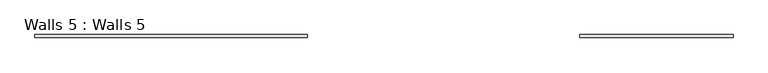
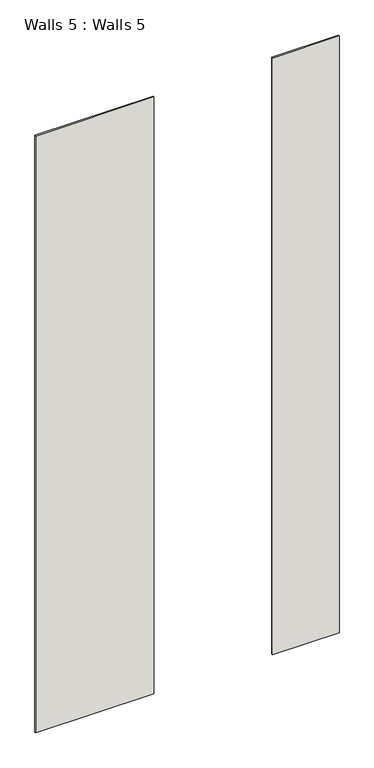
"""IFC4 building model written with IfcOpenShell, lengths in millimetres: wall geometry, Walls 5 : Walls 5."""

from ifc_helpers import new_model, si_unit, frame, origin, place, context, project, spatial, polyline, outline, extrude, source, transform, mapped, element, save


def walls_5_walls_5_43feafce(model_context):
    return source(origin(), model_context, "Body", "SweptSolid", [
        extrude(outline(polyline([(3838.3430349, 426.1055142), (2517.5430349, 426.1055142), (2517.5430349, 451.5055142), (3838.3430349, 451.5055142), (3838.3430349, 426.1055142)])), frame((0.0, 0.0, 2743.2), z_axis=(0.0, 0.0, 1.0), x_axis=(1.0, 0.0, 0.0)), (0.0, 0.0, 1.0), 12490.45),
        extrude(outline(polyline([(172.3175011, 426.1055142), (-2168.7569651, 426.1055142), (-2168.7569651, 451.5055142), (172.3175011, 451.5055142), (172.3175011, 426.1055142)])), frame((0.0, 0.0, 2747.0724171), z_axis=(0.0, 0.0, 1.0), x_axis=(1.0, 0.0, 0.0)), (0.0, 0.0, 1.0), 12492.9275829),
    ])


if __name__ == "__main__":
    model = new_model("IFC4")
    model_context = context("Model", 3, world=origin())
    ifc_project = project(units=[si_unit("LENGTHUNIT", "METRE", prefix="MILLI")], contexts=[model_context])
    site = spatial("IfcSite", under=ifc_project)
    building = spatial("IfcBuilding", under=site)
    placement = place(None, origin())
    walls_5_walls_5_shape = walls_5_walls_5_43feafce(model_context)
    element("IfcWall", 1, ObjectType="Walls 5 : Walls 5", at=placement, inside=building, context=model_context, shape_type="MappedRepresentation", body=[
        mapped(walls_5_walls_5_shape, transform((0.0, 0.0, 0.0), x_axis=(1.0, 0.0, 0.0), y_axis=(0.0, 1.0, 0.0), z_axis=(0.0, 0.0, 1.0))),
    ])
    save(model, "model.ifc")

# Revit data of these elements
# Element 1 (IfcWall, "Walls 5 : Walls 5")
#   Materials on its faces: "Default Wall", "1 wall white"
# Materials
#   "Default Wall": colour RGB 128 128 128, transparency 0, Cost = 0
#   "1 wall white": class "Generic", colour RGB 244 245 241, transparency 0, Cost = 0
